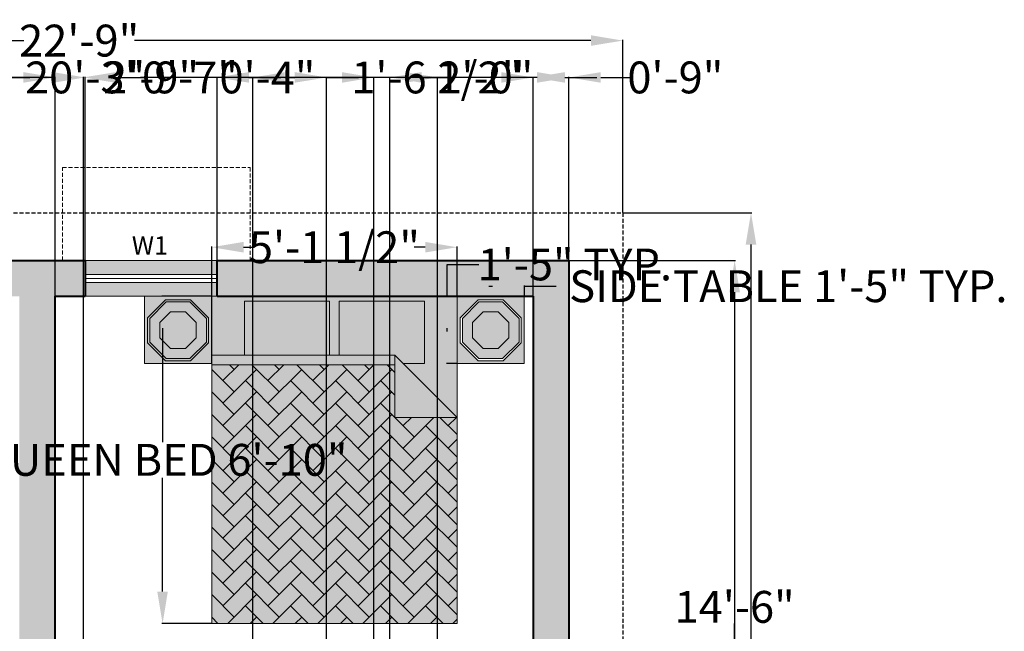
# Model space of a CAD drawing. Units: inches. Extents: x 277 to 728, y 649 to 1132.
# Tile 4 of 4: x 447 to 694, y 978 to 1132. Entities that reach past the tile are written whole.
import ezdxf

# ---------------------------------------------------------------- set-up
doc = ezdxf.new("R2010")
doc.units = ezdxf.units.IN
doc.header["$MEASUREMENT"] = 0
doc.linetypes.add('DASHEDX2', pattern=[1.5, 1, -0.5])
for name, color, linetype, lineweight in [('A-ANNO-DIMS', 2, 'Continuous', 18), ('A-ANNO-TEXT', 7, 'Continuous', 18), ('A-FURN', 8, 'Continuous', 18), ('A-FURN-TXTR-PATT', 7, 'Continuous', 9), ('A-GLAZ', 4, 'Continuous', 18), ('A-GLAZ-OVHD', 8, 'DASHEDX2', 13), ('A-WALL', 7, 'Continuous', 40), ('A-WALL-PATT', 8, 'Continuous', 13), ('C-PROP', 7, 'DASHEDX2', 25)]:
    doc.layers.add(name, color=color, linetype=linetype, lineweight=lineweight)
doc.layers.add('A-FURN-PATT', color=9, linetype='Continuous', lineweight=9, true_color=0xd6bdce)
doc.layers.add('A-GLAZ-PATT', color=144, linetype='Continuous', lineweight=13, true_color=0x1e788f)
doc.styles.get("Standard").update_dxf_attribs({"font": 'arial.ttf'})
doc.dimstyles.get("Standard").update_dxf_attribs({"dimtxt": 8, "dimasz": 8, "dimexe": 0.18, "dimexo": 0.0625, "dimgap": 0.09, "dimtad": 0, "dimtih": 1, "dimtoh": 1, "dimdec": 0, "dimzin": 0, "dimdsep": 46, "dimlunit": 3, "dimtxsty": 'Standard', "dimcen": 0.09, "dimadec": 0, "dimazin": 0, "dimtfac": 1, "dimtdec": 0, "dimtofl": 0, "dimtmove": 0, "dimatfit": 3, "dimfxl": 1, "dimtolj": 1, "dimtzin": 0, "dimarcsym": 0})

# ---------------------------------------------------------------- blocks, each defined once
blk = doc.blocks.new('Bed - Queen')
for p, q in [((0, -80.00003), (0, 0)), ((0, 0), (59.99999, 0)), ((59.99999, 0), (59.99999, -80.00003)), ((7.99999, -1.2), (28.79998, -1.2)), ((7.99999, -14.4), (7.99999, -1.2)), ((28.79998, -1.2), (28.79998, -14.4)), ((31.19999, -1.2), (51.99999, -1.2)), ((31.19999, -14.4), (31.19999, -1.2)), ((51.99999, -1.2), (51.99999, -16.4)), ((0, -14.4), (44.8, -14.4)), ((59.99999, -29.6), (44.8, -14.4)), ((44.8, -14.4), (44.8, -29.6)), ((44.8, -16.8), (0, -16.8)), ((51.99999, -16.4), (46.79936, -16.4)), ((44.8, -29.6), (59.99999, -29.6)), ((59.99999, -80.00003), (0, -80.00003))]:
    blk.add_line(p, q)
blk = doc.blocks.new('Hot Tub')
for p, q in [((0, 0), (0, 69.12)), ((0, 69.12), (69.12, 69.12)), ((21.601, 65.456), (3.272, 47.128)), ((22.464, 63.396), (5.358, 46.29)), ((47.521, 65.456), (21.601, 65.456)), ((46.656, 63.396), (22.464, 63.396)), ((63.763, 46.29), (46.656, 63.396)), ((65.849, 47.128), (47.521, 65.456)), ((69.12, 69.12), (69.12, 0)), ((26.785, 53.097), (15.788, 42.101)), ((42.337, 53.097), (26.785, 53.097)), ((53.333, 42.101), (42.337, 53.097)), ((3.272, 47.128), (3.272, 21.208)), ((5.358, 46.29), (5.358, 22.098)), ((15.788, 42.101), (15.788, 26.549)), ((53.333, 26.549), (53.333, 42.101)), ((63.763, 22.098), (63.763, 46.29)), ((65.849, 21.208), (65.849, 47.128)), ((3.272, 21.208), (21.601, 2.88)), ((5.358, 22.098), (22.464, 4.992)), ((15.788, 26.549), (26.785, 15.552)), ((42.337, 15.552), (53.333, 26.549)), ((46.656, 4.992), (63.763, 22.098)), ((47.521, 2.88), (65.849, 21.208)), ((26.785, 15.552), (42.337, 15.552)), ((69.12, 0), (0, 0)), ((21.601, 2.88), (47.521, 2.88)), ((22.464, 4.992), (46.656, 4.992))]:
    blk.add_line(p, q)
blk = doc.blocks.new('*D20')
at = {"layer": 'A-ANNO-DIMS', "color": 0, "lineweight": -2, "transparency": 16777216}
for p, q in [((325.22, 1083.11), (325.22, 1126.48)), ((333.22, 1126.3), (447.82, 1126.3)), ((590.22, 1126.3), (475.62, 1126.3)), ((598.22, 1083.11), (598.22, 1126.48))]:
    blk.add_line(p, q, dxfattribs=at)
at = {"layer": 'A-ANNO-DIMS', "color": 0, "transparency": 16777216}
for points in [[(333.22, 1127.64), (333.22, 1124.97), (325.22, 1126.3)], [(590.22, 1127.64), (590.22, 1124.97), (598.22, 1126.3)]]:
    blk.add_solid(points, dxfattribs=at)
at = {"layer": 'Defpoints', "color": 0, "transparency": 16777216}
for p in [(598.22, 1126.3), (325.22, 1083.05), (598.22, 1083.05)]:
    blk.add_point(p, dxfattribs=at)
at = {"layer": 'A-ANNO-DIMS', "color": 0, "transparency": 16777216, "insert": (461.72, 1126.3), "char_height": 8, "attachment_point": 5}
blk.add_mtext('\\A1;22\'-9"', dxfattribs=at)
blk = doc.blocks.new('*D21')
at = {"layer": 'A-ANNO-DIMS', "color": 0, "lineweight": -2, "transparency": 16777216}
for p, q in [((598.28, 1083.05), (630.62, 1083.05)), ((630.44, 1075.05), (630.44, 907.23)), ((630.44, 731.05), (630.44, 898.87)), ((598.28, 723.05), (630.62, 723.05))]:
    blk.add_line(p, q, dxfattribs=at)
at = {"layer": 'A-ANNO-DIMS', "color": 0, "transparency": 16777216}
for points in [[(629.11, 1075.05), (631.77, 1075.05), (630.44, 1083.05)], [(629.11, 731.05), (631.77, 731.05), (630.44, 723.05)]]:
    blk.add_solid(points, dxfattribs=at)
at = {"layer": 'Defpoints', "color": 0, "transparency": 16777216}
for p in [(598.22, 1083.05), (598.22, 723.05), (630.44, 723.05)]:
    blk.add_point(p, dxfattribs=at)
at = {"layer": 'A-ANNO-DIMS', "color": 0, "transparency": 16777216, "insert": (630.44, 903.05), "char_height": 8, "attachment_point": 5}
blk.add_mtext("\\A1;30'", dxfattribs=at)
blk = doc.blocks.new('*D23')
at = {"layer": 'A-ANNO-DIMS', "color": 0, "lineweight": -2, "transparency": 16777216}
for p, q in [((556.64, 1062.11), (556.64, 1064.76)), ((564.64, 1064.58), (565.52, 1064.58)), ((573.52, 1062.11), (573.52, 1064.76)), ((573.52, 1064.58), (581.52, 1064.58))]:
    blk.add_line(p, q, dxfattribs=at)
at = {"layer": 'A-ANNO-DIMS', "color": 0, "transparency": 16777216}
for points in [[(564.64, 1065.92), (564.64, 1063.25), (556.64, 1064.58)], [(565.52, 1065.92), (565.52, 1063.25), (573.52, 1064.58)]]:
    blk.add_solid(points, dxfattribs=at)
at = {"layer": 'Defpoints', "color": 0, "transparency": 16777216}
for p in [(573.52, 1064.58), (556.64, 1062.05), (573.52, 1062.05)]:
    blk.add_point(p, dxfattribs=at)
at = {"layer": 'A-ANNO-DIMS', "color": 0, "transparency": 16777216, "insert": (639.82, 1064.58), "char_height": 8, "attachment_point": 5}
blk.add_mtext('\\A1;SIDE TABLE 1\'-5" TYP.', dxfattribs=at)
blk = doc.blocks.new('*D24')
at = {"layer": 'A-ANNO-DIMS', "color": 0, "lineweight": -2, "transparency": 16777216}
for p, q in [((554.11, 1062.05), (554.11, 1070.05)), ((554.11, 1070.05), (562.11, 1070.05)), ((556.58, 1062.05), (553.93, 1062.05)), ((554.11, 1053.17), (554.11, 1054.05)), ((556.58, 1045.17), (553.93, 1045.17))]:
    blk.add_line(p, q, dxfattribs=at)
at = {"layer": 'A-ANNO-DIMS', "color": 0, "transparency": 16777216}
for points in [[(552.78, 1054.05), (555.44, 1054.05), (554.11, 1062.05)], [(552.78, 1053.17), (555.44, 1053.17), (554.11, 1045.17)]]:
    blk.add_solid(points, dxfattribs=at)
at = {"layer": 'Defpoints', "color": 0, "transparency": 16777216}
for p in [(554.11, 1062.05), (556.64, 1062.05), (556.64, 1045.17)]:
    blk.add_point(p, dxfattribs=at)
at = {"layer": 'A-ANNO-DIMS', "color": 0, "transparency": 16777216, "insert": (586.2, 1070.05), "char_height": 8, "attachment_point": 5}
blk.add_mtext('\\A1;1\'-5" TYP.', dxfattribs=at)
blk = doc.blocks.new('*D37')
at = {"layer": 'A-ANNO-DIMS', "color": 0, "lineweight": -2, "transparency": 16777216}
for p, q in [((494.94, 1062.05), (482.49, 1062.05)), ((482.67, 1054.05), (482.67, 1025.43)), ((482.67, 987.86), (482.67, 1016.48)), ((494.94, 979.86), (482.49, 979.86))]:
    blk.add_line(p, q, dxfattribs=at)
at = {"layer": 'A-ANNO-DIMS', "color": 0, "transparency": 16777216}
for points in [[(481.34, 1054.05), (484, 1054.05), (482.67, 1062.05)], [(481.34, 987.86), (484, 987.86), (482.67, 979.86)]]:
    blk.add_solid(points, dxfattribs=at)
at = {"layer": 'Defpoints', "color": 0, "transparency": 16777216}
for p in [(482.67, 1062.05), (495, 1062.05), (495, 979.86)]:
    blk.add_point(p, dxfattribs=at)
at = {"layer": 'A-ANNO-DIMS', "color": 0, "transparency": 16777216, "insert": (482.67, 1020.96), "char_height": 8, "attachment_point": 5}
blk.add_mtext('\\A1;QUEEN BED 6\'-10"', dxfattribs=at)
blk = doc.blocks.new('*D38')
at = {"layer": 'A-ANNO-DIMS', "color": 0, "lineweight": -2, "transparency": 16777216}
for p, q in [((495, 1062.11), (495, 1074.56)), ((503, 1074.38), (505.78, 1074.38)), ((548.64, 1074.38), (545.86, 1074.38)), ((556.64, 1062.11), (556.64, 1074.56))]:
    blk.add_line(p, q, dxfattribs=at)
at = {"layer": 'A-ANNO-DIMS', "color": 0, "transparency": 16777216}
for points in [[(503, 1075.71), (503, 1073.05), (495, 1074.38)], [(548.64, 1075.71), (548.64, 1073.05), (556.64, 1074.38)]]:
    blk.add_solid(points, dxfattribs=at)
at = {"layer": 'Defpoints', "color": 0, "transparency": 16777216}
for p in [(556.64, 1074.38), (495, 1062.05), (556.64, 1062.05)]:
    blk.add_point(p, dxfattribs=at)
at = {"layer": 'A-ANNO-DIMS', "color": 0, "transparency": 16777216, "insert": (525.82, 1074.38), "char_height": 8, "attachment_point": 5}
blk.add_mtext('\\A1;5\'-1 1/2"', dxfattribs=at)
blk = doc.blocks.new('*D42')
at = {"layer": 'A-ANNO-DIMS', "color": 0, "lineweight": -2, "transparency": 16777216}
for p, q in [((505.35, 907.07), (505.35, 1117.22)), ((513.35, 1117.04), (515.86, 1117.04)), ((523.86, 907.07), (523.86, 1117.22)), ((523.86, 1117.04), (531.86, 1117.04))]:
    blk.add_line(p, q, dxfattribs=at)
at = {"layer": 'A-ANNO-DIMS', "color": 0, "transparency": 16777216}
for points in [[(513.35, 1118.37), (513.35, 1115.71), (505.35, 1117.04)], [(515.86, 1118.37), (515.86, 1115.71), (523.86, 1117.04)]]:
    blk.add_solid(points, dxfattribs=at)
at = {"layer": 'Defpoints', "color": 0, "transparency": 16777216}
for p in [(523.86, 1117.04), (505.35, 907.01), (523.86, 907.01)]:
    blk.add_point(p, dxfattribs=at)
at = {"layer": 'A-ANNO-DIMS', "color": 0, "transparency": 16777216, "insert": (551.53, 1117.04), "char_height": 8, "attachment_point": 5}
blk.add_mtext('\\A1;1\'-6 1/2"', dxfattribs=at)
blk = doc.blocks.new('*D44')
at = {"layer": 'A-ANNO-DIMS', "color": 0, "lineweight": -2, "transparency": 16777216}
for p, q in [((543.72, 1117.04), (535.72, 1117.04)), ((551.72, 844.96), (551.72, 1117.22)), ((575.72, 844.96), (575.72, 1117.22)), ((583.72, 1117.04), (591.72, 1117.04))]:
    blk.add_line(p, q, dxfattribs=at)
at = {"layer": 'A-ANNO-DIMS', "color": 0, "transparency": 16777216}
for points in [[(543.72, 1118.37), (543.72, 1115.71), (551.72, 1117.04)], [(583.72, 1118.37), (583.72, 1115.71), (575.72, 1117.04)]]:
    blk.add_solid(points, dxfattribs=at)
at = {"layer": 'Defpoints', "color": 0, "transparency": 16777216}
for p in [(575.72, 1117.04), (551.72, 844.9), (575.72, 844.9)]:
    blk.add_point(p, dxfattribs=at)
at = {"layer": 'A-ANNO-DIMS', "color": 0, "transparency": 16777216, "insert": (563.72, 1117.04), "char_height": 8, "attachment_point": 5}
blk.add_mtext('\\A1;2\'-0"', dxfattribs=at)
blk = doc.blocks.new('*D47')
at = {"layer": 'A-ANNO-DIMS', "color": 0, "lineweight": -2, "transparency": 16777216}
for p, q in [((341.72, 1071.11), (341.72, 1117.22)), ((349.72, 1117.04), (449.32, 1117.04)), ((576.72, 1117.04), (477.12, 1117.04)), ((584.72, 1071.11), (584.72, 1117.22))]:
    blk.add_line(p, q, dxfattribs=at)
at = {"layer": 'A-ANNO-DIMS', "color": 0, "transparency": 16777216}
for points in [[(349.72, 1118.37), (349.72, 1115.71), (341.72, 1117.04)], [(576.72, 1118.37), (576.72, 1115.71), (584.72, 1117.04)]]:
    blk.add_solid(points, dxfattribs=at)
at = {"layer": 'Defpoints', "color": 0, "transparency": 16777216}
for p in [(584.72, 1117.04), (341.72, 1071.05), (584.72, 1071.05)]:
    blk.add_point(p, dxfattribs=at)
at = {"layer": 'A-ANNO-DIMS', "color": 0, "transparency": 16777216, "insert": (463.22, 1117.04), "char_height": 8, "attachment_point": 5}
blk.add_mtext('\\A1;20\'-3"', dxfattribs=at)
blk = doc.blocks.new('*D48')
at = {"layer": 'A-ANNO-DIMS', "color": 0, "lineweight": -2, "transparency": 16777216}
for p, q in [((584.78, 1071.05), (626.51, 1071.05)), ((626.33, 1063.05), (626.33, 901.23)), ((626.33, 731.05), (626.33, 892.88)), ((584.78, 723.05), (626.51, 723.05))]:
    blk.add_line(p, q, dxfattribs=at)
at = {"layer": 'A-ANNO-DIMS', "color": 0, "transparency": 16777216}
for points in [[(625, 1063.05), (627.67, 1063.05), (626.33, 1071.05)], [(625, 731.05), (627.67, 731.05), (626.33, 723.05)]]:
    blk.add_solid(points, dxfattribs=at)
at = {"layer": 'Defpoints', "color": 0, "transparency": 16777216}
for p in [(584.72, 1071.05), (626.33, 1071.05), (584.72, 723.05)]:
    blk.add_point(p, dxfattribs=at)
at = {"layer": 'A-ANNO-DIMS', "color": 0, "transparency": 16777216, "insert": (626.33, 897.05), "char_height": 8, "attachment_point": 5}
blk.add_mtext('\\A1;29\'-0"', dxfattribs=at)
blk = doc.blocks.new('*D49')
at = {"layer": 'A-ANNO-DIMS', "color": 0, "lineweight": -2, "transparency": 16777216}
for p, q in [((341.72, 1071.11), (341.72, 1117.22)), ((349.72, 1117.04), (379.69, 1117.04)), ((455.22, 1117.04), (425.24, 1117.04)), ((463.22, 1071.11), (463.22, 1117.22))]:
    blk.add_line(p, q, dxfattribs=at)
at = {"layer": 'A-ANNO-DIMS', "color": 0, "transparency": 16777216}
for points in [[(349.72, 1118.37), (349.72, 1115.71), (341.72, 1117.04)], [(455.22, 1118.37), (455.22, 1115.71), (463.22, 1117.04)]]:
    blk.add_solid(points, dxfattribs=at)
at = {"layer": 'Defpoints', "color": 0, "transparency": 16777216}
for p in [(463.22, 1117.04), (341.72, 1071.05), (463.22, 1071.05)]:
    blk.add_point(p, dxfattribs=at)
at = {"layer": 'A-ANNO-DIMS', "color": 0, "transparency": 16777216, "insert": (402.47, 1117.04), "char_height": 8, "attachment_point": 5}
blk.add_mtext('\\A1;10\'-1 1/2"', dxfattribs=at)
blk = doc.blocks.new('*D50')
at = {"layer": 'A-ANNO-DIMS', "color": 0, "lineweight": -2, "transparency": 16777216}
for p, q in [((455.22, 1117.04), (447.22, 1117.04)), ((463.22, 1071.11), (463.22, 1117.22)), ((496.36, 1071.11), (496.36, 1117.22)), ((504.36, 1117.04), (512.36, 1117.04))]:
    blk.add_line(p, q, dxfattribs=at)
at = {"layer": 'A-ANNO-DIMS', "color": 0, "transparency": 16777216}
for points in [[(455.22, 1118.37), (455.22, 1115.71), (463.22, 1117.04)], [(504.36, 1118.37), (504.36, 1115.71), (496.36, 1117.04)]]:
    blk.add_solid(points, dxfattribs=at)
at = {"layer": 'Defpoints', "color": 0, "transparency": 16777216}
for p in [(496.36, 1117.04), (463.22, 1071.05), (496.36, 1071.05)]:
    blk.add_point(p, dxfattribs=at)
at = {"layer": 'A-ANNO-DIMS', "color": 0, "transparency": 16777216, "insert": (479.79, 1117.04), "char_height": 8, "attachment_point": 5}
blk.add_mtext('\\A1;2\'-9"', dxfattribs=at)
blk = doc.blocks.new('*D54')
at = {"layer": 'A-ANNO-DIMS', "color": 0, "lineweight": -2, "transparency": 16777216}
for p, q in [((584.78, 1071.05), (626.51, 1071.05)), ((626.33, 1063.05), (626.33, 988.2)), ((626.33, 905), (626.33, 979.85)), ((584.78, 897), (626.51, 897))]:
    blk.add_line(p, q, dxfattribs=at)
at = {"layer": 'A-ANNO-DIMS', "color": 0, "transparency": 16777216}
for points in [[(625, 1063.05), (627.67, 1063.05), (626.33, 1071.05)], [(625, 905), (627.67, 905), (626.33, 897)]]:
    blk.add_solid(points, dxfattribs=at)
at = {"layer": 'Defpoints', "color": 0, "transparency": 16777216}
for p in [(584.72, 1071.05), (626.33, 1071.05), (584.72, 897)]:
    blk.add_point(p, dxfattribs=at)
at = {"layer": 'A-ANNO-DIMS', "color": 0, "transparency": 16777216, "insert": (626.33, 984.02), "char_height": 8, "attachment_point": 5}
blk.add_mtext('\\A1;14\'-6"', dxfattribs=at)
blk = doc.blocks.new('*D65')
at = {"layer": 'A-ANNO-DIMS', "color": 0, "lineweight": -2, "transparency": 16777216}
for p, q in [((447.72, 1117.04), (439.72, 1117.04)), ((455.72, 942.11), (455.72, 1117.22)), ((462.81, 942.11), (462.81, 1117.22)), ((470.81, 1117.04), (478.81, 1117.04))]:
    blk.add_line(p, q, dxfattribs=at)
at = {"layer": 'A-ANNO-DIMS', "color": 0, "transparency": 16777216}
for points in [[(447.72, 1118.37), (447.72, 1115.71), (455.72, 1117.04)], [(470.81, 1118.37), (470.81, 1115.71), (462.81, 1117.04)]]:
    blk.add_solid(points, dxfattribs=at)
at = {"layer": 'Defpoints', "color": 0, "transparency": 16777216}
for p in [(462.81, 1117.04), (455.72, 942.05), (462.81, 942.05)]:
    blk.add_point(p, dxfattribs=at)
at = {"layer": 'A-ANNO-DIMS', "color": 0, "transparency": 16777216, "insert": (489.54, 1117.04), "char_height": 8, "attachment_point": 5}
blk.add_mtext('\\A1;0\'-7"', dxfattribs=at)
blk = doc.blocks.new('*D73')
at = {"layer": 'A-ANNO-DIMS', "color": 0, "lineweight": -2, "transparency": 16777216}
for p, q in [((567.72, 1117.04), (559.72, 1117.04)), ((575.72, 1062.11), (575.72, 1117.22)), ((584.72, 1071.11), (584.72, 1117.22)), ((592.72, 1117.04), (600.72, 1117.04))]:
    blk.add_line(p, q, dxfattribs=at)
at = {"layer": 'A-ANNO-DIMS', "color": 0, "transparency": 16777216}
for points in [[(567.72, 1118.37), (567.72, 1115.71), (575.72, 1117.04)], [(592.72, 1118.37), (592.72, 1115.71), (584.72, 1117.04)]]:
    blk.add_solid(points, dxfattribs=at)
at = {"layer": 'Defpoints', "color": 0, "transparency": 16777216}
for p in [(584.72, 1117.04), (584.72, 1071.05), (575.72, 1062.05)]:
    blk.add_point(p, dxfattribs=at)
at = {"layer": 'A-ANNO-DIMS', "color": 0, "transparency": 16777216, "insert": (611.44, 1117.04), "char_height": 8, "attachment_point": 5}
blk.add_mtext('\\A1;0\'-9"', dxfattribs=at)
blk = doc.blocks.new('*D75')
at = {"layer": 'A-ANNO-DIMS', "color": 0, "lineweight": -2, "transparency": 16777216}
for p, q in [((527.72, 1117.04), (519.72, 1117.04)), ((535.72, 784.69), (535.72, 1117.22)), ((539.72, 784.69), (539.72, 1117.22)), ((547.72, 1117.04), (555.72, 1117.04))]:
    blk.add_line(p, q, dxfattribs=at)
at = {"layer": 'A-ANNO-DIMS', "color": 0, "transparency": 16777216}
for points in [[(527.72, 1118.37), (527.72, 1115.71), (535.72, 1117.04)], [(547.72, 1118.37), (547.72, 1115.71), (539.72, 1117.04)]]:
    blk.add_solid(points, dxfattribs=at)
at = {"layer": 'Defpoints', "color": 0, "transparency": 16777216}
for p in [(535.72, 1117.04), (535.72, 784.62), (539.72, 784.62)]:
    blk.add_point(p, dxfattribs=at)
at = {"layer": 'A-ANNO-DIMS', "color": 0, "transparency": 16777216, "insert": (509, 1117.04), "char_height": 8, "attachment_point": 5}
blk.add_mtext('\\A1;0\'-4"', dxfattribs=at)

msp = doc.modelspace()

# ---------------------------------------------------------------- hatches: boundary and pattern name
at = {"layer": 'A-FURN-PATT'}
h = msp.add_hatch(color=256, dxfattribs=at)
h.dxf.hatch_style = 1
h.paths.add_polyline_path([(495, 1045.17), (495, 1062.05), (478.12, 1062.05), (478.12, 1045.17)])
h.paths.add_polyline_path([(489.72, 1045.88), (483.4, 1045.88), (478.92, 1050.35), (478.92, 1056.68), (483.4, 1061.16), (489.72, 1061.16), (494.2, 1056.68), (494.2, 1050.35)], flags=16)
h.paths.add_polyline_path([(489.51, 1046.39), (483.61, 1046.39), (479.43, 1050.57), (479.43, 1056.48), (483.61, 1060.65), (489.51, 1060.65), (493.69, 1056.48), (493.69, 1050.57)], flags=0)
h.paths.add_polyline_path([(488.46, 1048.97), (484.66, 1048.97), (481.98, 1051.66), (481.98, 1055.45), (484.66, 1058.14), (488.46, 1058.14), (491.14, 1055.45), (491.14, 1051.66)], flags=0)
h = msp.add_hatch(color=256, dxfattribs=at)
h.dxf.hatch_style = 1
h.paths.add_polyline_path([(493.69, 1050.57), (493.69, 1056.48), (489.51, 1060.65), (483.61, 1060.65), (479.43, 1056.48), (479.43, 1050.57), (483.61, 1046.39), (489.51, 1046.39)], flags=16)
h.paths.add_polyline_path([(494.2, 1050.35), (494.2, 1056.68), (489.72, 1061.16), (483.4, 1061.16), (478.92, 1056.68), (478.92, 1050.35), (483.4, 1045.88), (489.72, 1045.88)])
h = msp.add_hatch(color=256, dxfattribs=at)
h.dxf.hatch_style = 1
h.paths.add_polyline_path([(493.69, 1050.57), (493.69, 1056.48), (489.51, 1060.65), (483.61, 1060.65), (479.43, 1056.48), (479.43, 1050.57), (483.61, 1046.39), (489.51, 1046.39)], flags=16)
h.paths.add_polyline_path([(494.2, 1050.35), (494.2, 1056.68), (489.72, 1061.16), (483.4, 1061.16), (478.92, 1056.68), (478.92, 1050.35), (483.4, 1045.88), (489.72, 1045.88)])
h = msp.add_hatch(color=256, dxfattribs=at)
h.dxf.hatch_style = 1
h.paths.add_polyline_path([(556.64, 1031.64), (556.64, 1062.05), (495, 1062.05), (495, 1047.26), (503.22, 1047.26), (503.22, 1060.82), (524.59, 1060.82), (524.59, 1047.26), (527.05, 1047.26), (527.05, 1060.82), (548.42, 1060.82), (548.42, 1045.2), (543.08, 1045.2)])
h = msp.add_hatch(color=256, dxfattribs=at)
h.dxf.hatch_style = 1
h.paths.add_polyline_path([(503.22, 1060.82), (503.22, 1047.26), (524.59, 1047.26), (524.59, 1060.82)])
h = msp.add_hatch(color=256, dxfattribs=at)
h.dxf.hatch_style = 1
h.paths.add_polyline_path([(527.05, 1047.26), (541.02, 1047.26), (543.08, 1045.2), (548.42, 1045.2), (548.42, 1060.82), (527.05, 1060.82)])
h = msp.add_hatch(color=256, dxfattribs=at)
h.dxf.hatch_style = 1
h.paths.add_polyline_path([(573.52, 1062.05), (556.64, 1062.05), (556.64, 1045.17), (573.52, 1045.17)])
h.paths.add_polyline_path([(557.44, 1050.35), (557.44, 1056.68), (561.92, 1061.16), (568.24, 1061.16), (572.72, 1056.68), (572.72, 1050.35), (568.24, 1045.88), (561.92, 1045.88)], flags=16)
h.paths.add_polyline_path([(557.95, 1050.57), (557.95, 1056.48), (562.13, 1060.65), (568.03, 1060.65), (572.21, 1056.48), (572.21, 1050.57), (568.03, 1046.39), (562.13, 1046.39)], flags=0)
h.paths.add_polyline_path([(560.5, 1051.66), (560.5, 1055.45), (563.18, 1058.14), (566.98, 1058.14), (569.66, 1055.45), (569.66, 1051.66), (566.98, 1048.97), (563.18, 1048.97)], flags=0)
h = msp.add_hatch(color=256, dxfattribs=at)
h.dxf.hatch_style = 1
h.paths.add_polyline_path([(489.51, 1046.39), (493.69, 1050.57), (493.69, 1056.48), (489.51, 1060.65), (483.61, 1060.65), (479.43, 1056.48), (479.43, 1050.57), (483.61, 1046.39)])
h.paths.add_polyline_path([(484.66, 1048.97), (481.98, 1051.66), (481.98, 1055.45), (484.66, 1058.14), (488.46, 1058.14), (491.14, 1055.45), (491.14, 1051.66), (488.46, 1048.97)], flags=16)
h = msp.add_hatch(color=256, dxfattribs=at)
h.dxf.hatch_style = 1
h.paths.add_polyline_path([(563.18, 1048.97), (566.98, 1048.97), (569.66, 1051.66), (569.66, 1055.45), (566.98, 1058.14), (563.18, 1058.14), (560.5, 1055.45), (560.5, 1051.66)], flags=16)
h.paths.add_polyline_path([(562.13, 1046.39), (568.03, 1046.39), (572.21, 1050.57), (572.21, 1056.48), (568.03, 1060.65), (562.13, 1060.65), (557.95, 1056.48), (557.95, 1050.57)])
h = msp.add_hatch(color=256, dxfattribs=at)
h.dxf.hatch_style = 1
h.paths.add_polyline_path([(491.14, 1051.66), (491.14, 1055.45), (488.46, 1058.14), (484.66, 1058.14), (481.98, 1055.45), (481.98, 1051.66), (484.66, 1048.97), (488.46, 1048.97)])
h = msp.add_hatch(color=256, dxfattribs=at)
h.dxf.hatch_style = 1
h.paths.add_polyline_path([(563.18, 1048.97), (566.98, 1048.97), (569.66, 1051.66), (569.66, 1055.45), (566.98, 1058.14), (563.18, 1058.14), (560.5, 1055.45), (560.5, 1051.66)])
h = msp.add_hatch(color=256, dxfattribs=at)
h.dxf.hatch_style = 1
h.paths.add_polyline_path([(495, 1047.26), (495, 1044.79), (541.02, 1044.79), (541.02, 1047.26)])
h = msp.add_hatch(color=256, dxfattribs=at)
h.dxf.hatch_style = 1
h.paths.add_polyline_path([(541.02, 1031.64), (556.64, 1031.64), (541.02, 1047.26)])
h = msp.add_hatch(color=256, dxfattribs=at)
h.dxf.hatch_style = 1
h.paths.add_polyline_path([(495, 979.86), (556.64, 979.86), (556.64, 1031.64), (541.02, 1031.64), (541.02, 1044.79), (495, 1044.79)])
at = {"layer": 'A-FURN-TXTR-PATT'}
h = msp.add_hatch(dxfattribs=at)
h.set_pattern_fill('AR-HBONE', color=256)
h.paths.add_polyline_path([(556.64, 979.86), (556.64, 1031.64), (541.02, 1031.64), (541.02, 1044.79), (495, 1044.79), (495, 979.86)])
at = {"layer": 'A-GLAZ-PATT'}
h = msp.add_hatch(color=256, dxfattribs=at)
h.dxf.hatch_style = 1
h.paths.add_polyline_path([(496.36, 1067.55), (496.36, 1071.05), (463.22, 1071.05), (463.22, 1067.55)])
h = msp.add_hatch(color=256, dxfattribs=at)
h.dxf.hatch_style = 1
h.paths.add_polyline_path([(463.22, 1065.55), (463.22, 1062.05), (496.36, 1062.05), (496.36, 1065.55)])
at = {"layer": 'A-WALL-PATT'}
h = msp.add_hatch(color=256, dxfattribs=at)
h.dxf.hatch_style = 1
h.paths.add_polyline_path([(446.72, 942.05), (422.67, 942.05), (422.67, 933.05), (462.81, 933.05), (462.81, 942.05), (455.72, 942.05), (455.72, 1062.05), (463.22, 1062.05), (463.22, 1071.05), (341.72, 1071.05), (341.72, 981.3), (350.72, 981.3), (350.72, 1062.05), (446.72, 1062.05)])
h = msp.add_hatch(color=256, dxfattribs=at)
h.dxf.hatch_style = 1
h.paths.add_polyline_path([(544.2, 933.05), (575.72, 933.05), (575.72, 897), (584.72, 897), (584.72, 1071.05), (496.36, 1071.05), (496.36, 1062.05), (575.72, 1062.05), (575.72, 942.05), (492.89, 942.05), (492.89, 933.05)])

# ---------------------------------------------------------------- linework, layer by layer
at = {"layer": 'A-GLAZ'}
for p, q in [((463.22, 1071.05), (496.36, 1071.05)), ((463.22, 1067.55), (496.36, 1067.55)), ((463.22, 1066.55), (496.36, 1066.55)), ((463.22, 1065.55), (496.36, 1065.55)), ((463.22, 1062.05), (496.36, 1062.05))]:
    msp.add_line(p, q, dxfattribs=at)
at = {"layer": 'A-GLAZ-OVHD'}
for p, q in [((457.56, 1071.05), (457.56, 1094.44)), ((457.56, 1094.44), (504.66, 1094.44)), ((504.66, 1094.44), (504.66, 1071.05))]:
    msp.add_line(p, q, dxfattribs=at)
at = {"layer": 'A-WALL'}
for p, q in [((341.72, 1071.05), (463.22, 1071.05)), ((463.22, 1071.05), (463.22, 1062.05)), ((496.36, 1062.05), (496.36, 1071.05)), ((496.36, 1071.05), (584.72, 1071.05)), ((584.72, 1071.05), (584.72, 897)), ((455.72, 1062.05), (463.22, 1062.05)), ((455.72, 942.05), (455.72, 1062.05)), ((496.36, 1062.05), (575.72, 1062.05)), ((575.72, 1062.05), (575.72, 942.05))]:
    msp.add_line(p, q, dxfattribs=at)
at = {"layer": 'C-PROP'}
for p, q in [((325.22, 1083.05), (598.22, 1083.05)), ((598.22, 1083.05), (598.22, 723.05))]:
    msp.add_line(p, q, dxfattribs=at)

# ---------------------------------------------------------------- block references
at = {"layer": 'A-FURN'}
for name, p, xscale, yscale, zscale in [('Hot Tub', (478.12, 1045.17), 0.2441715575500086, 0.2441715575500086, 0.2441715575500086), ('Bed - Queen', (495, 1062.05), 1.027370470334092, 1.027370470334092, 1.027370470334092), ('Hot Tub', (556.64, 1045.17), 0.2441715575500086, 0.2441715575500086, 0.2441715575500086)]:
    msp.add_blockref(name, p, dxfattribs=dict(at, xscale=xscale, yscale=yscale, zscale=zscale))

# ---------------------------------------------------------------- texts
at = {"layer": 'A-ANNO-TEXT', "insert": (474.94, 1077.15), "char_height": 4.66, "attachment_point": 1}
msp.add_mtext_dynamic_manual_height_columns('W1', width=6.3557, gutter_width=23.3, heights=[0], dxfattribs=at)

# ---------------------------------------------------------------- dimensions: what is measured, and where the dimension line sits
at = {"layer": 'A-ANNO-DIMS'}
for base, p1, p2, override, picture, middle in [((598.22, 1126.3), (325.22, 1083.05), (598.22, 1083.05), {"dimclrd": 0, "dimclre": 0, "dimclrt": 0}, '*D20', (461.72, 1126.3)), ((463.22, 1117.04), (341.72, 1071.05), (463.22, 1071.05), {"dimdec": 1, "dimlfac": 1, "dimrnd": 0, "dimzin": 1, "dimdsep": 46, "dimlunit": 4, "dimfrac": 2}, '*D49', (402.47, 1117.04)), ((523.86, 1117.04), (505.35, 907.01), (523.86, 907.01), {"dimdec": 1, "dimlfac": 1, "dimrnd": 0, "dimzin": 1, "dimdsep": 46, "dimlunit": 4, "dimfrac": 2}, '*D42', (551.53, 1117.04)), ((584.72, 1117.04), (341.72, 1071.05), (584.72, 1071.05), {"dimdec": 1, "dimlfac": 1, "dimrnd": 0, "dimzin": 1, "dimdsep": 46, "dimlunit": 4, "dimfrac": 2}, '*D47', (463.22, 1117.04)), ((462.81, 1117.04), (455.72, 942.05), (462.81, 942.05), {"dimdec": 1, "dimlfac": 1, "dimrnd": 0, "dimzin": 1, "dimdsep": 46, "dimlunit": 4, "dimfrac": 2}, '*D65', (489.54, 1117.04)), ((496.36, 1117.04), (463.22, 1071.05), (496.36, 1071.05), {"dimdec": 1, "dimlfac": 1, "dimrnd": 0, "dimzin": 1, "dimdsep": 46, "dimlunit": 4, "dimfrac": 2}, '*D50', (479.79, 1117.04)), ((535.72, 1117.04), (539.72, 784.62), (535.72, 784.62), {"dimdec": 1, "dimlfac": 1, "dimrnd": 0, "dimzin": 1, "dimdsep": 46, "dimlunit": 4, "dimfrac": 2}, '*D75', (509, 1117.04)), ((575.72, 1117.04), (551.72, 844.9), (575.72, 844.9), {"dimdec": 1, "dimlfac": 1, "dimrnd": 0, "dimzin": 1, "dimdsep": 46, "dimlunit": 4, "dimfrac": 2}, '*D44', (563.72, 1117.04)), ((584.72, 1117.04), (575.72, 1062.05), (584.72, 1071.05), {"dimdec": 1, "dimlfac": 1, "dimrnd": 0, "dimzin": 1, "dimdsep": 46, "dimlunit": 4, "dimfrac": 2}, '*D73', (611.44, 1117.04)), ((556.64, 1074.38), (495, 1062.05), (556.64, 1062.05), {"dimdec": 1, "dimlfac": 1, "dimrnd": 0, "dimzin": 1, "dimdsep": 46, "dimlunit": 4, "dimfrac": 2}, '*D38', (525.82, 1074.38))]:
    dim = msp.add_linear_dim(base=base, p1=p1, p2=p2, dimstyle='Standard', override=override, dxfattribs=at)
    dim.commit()
    dim.dimension.update_dxf_attribs({"geometry": picture, "text_midpoint": middle})
dim = msp.add_linear_dim(base=(573.52, 1064.58), p1=(556.64, 1062.05), p2=(573.52, 1062.05), text='SIDE TABLE <> TYP.', dimstyle='Standard', override={"dimdec": 1, "dimlfac": 1, "dimrnd": 0, "dimzin": 1, "dimdsep": 46, "dimlunit": 4, "dimfrac": 2}, dxfattribs=at)
dim.commit()
dim.dimension.update_dxf_attribs({"geometry": '*D23', "text_midpoint": (639.82, 1064.58)})
for base, p1, p2, override, picture, middle in [((630.44, 723.05), (598.22, 1083.05), (598.22, 723.05), {"dimclrd": 0, "dimclre": 0, "dimclrt": 0}, '*D21', (630.44, 903.05)), ((626.33, 1071.05), (584.72, 723.05), (584.72, 1071.05), {"dimdec": 1, "dimlfac": 1, "dimrnd": 0, "dimzin": 1, "dimdsep": 46, "dimlunit": 4, "dimfrac": 2}, '*D48', (626.33, 897.05)), ((626.3327, 1071.0508), (584.7185, 896.9974), (584.7185, 1071.0508), {"dimdec": 1, "dimlfac": 1, "dimrnd": 0, "dimzin": 1, "dimdsep": 46, "dimlunit": 4, "dimfrac": 2}, '*D54', (626.3327, 984.0241))]:
    dim = msp.add_linear_dim(base=base, p1=p1, p2=p2, angle=90, dimstyle='Standard', override=override, dxfattribs=at)
    dim.commit()
    dim.dimension.update_dxf_attribs({"geometry": picture, "text_midpoint": middle})
for base, p1, p2, text, picture, middle in [((554.11, 1062.05), (556.64, 1045.17), (556.64, 1062.05), '<> TYP.', '*D24', (586.2, 1070.05)), ((482.67, 1062.05), (495, 979.86), (495, 1062.05), 'QUEEN BED <>', '*D37', (482.67, 1020.96))]:
    dim = msp.add_linear_dim(base=base, p1=p1, p2=p2, angle=90, text=text, dimstyle='Standard', override={"dimdec": 1, "dimlfac": 1, "dimrnd": 0, "dimzin": 1, "dimdsep": 46, "dimlunit": 4, "dimfrac": 2}, dxfattribs=at)
    dim.commit()
    dim.dimension.update_dxf_attribs({"geometry": picture, "text_midpoint": middle})

doc.saveas('drawing.dxf')
